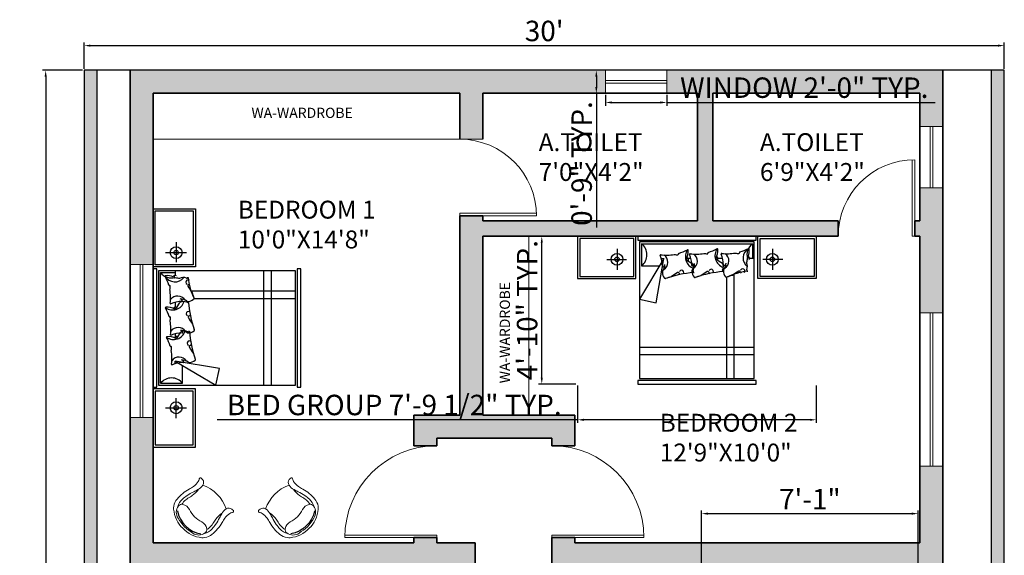
# Model space of a CAD drawing. Units: inches. Extents: x 2700 to 4052, y 1030 to 1872.
# Tile 4 of 8: x 2789 to 3175, y 1632 to 1841. Entities that reach past the tile are written whole.
import ezdxf

# ---------------------------------------------------------------- set-up
doc = ezdxf.new("R2010")
doc.units = ezdxf.units.IN
for name, color, linetype, lineweight in [('A-ANNO-DIMS', 2, 'Continuous', 13), ('A-ANNO-TEXT', 7, 'Continuous', 18), ('A-AREA-IDEN', 7, 'Continuous', 18), ('A-DOOR', 4, 'Continuous', 18), ('A-FLOR-CASE', 8, 'Continuous', 18), ('A-FURN', 8, 'Continuous', 18), ('A-GLAZ', 4, 'Continuous', 18), ('A-WALL', 7, 'Continuous', 35), ('A-WALL-PATT', 7, 'Continuous', 13), ('C-PROP', 7, 'Continuous', 25)]:
    doc.layers.add(name, color=color, linetype=linetype, lineweight=lineweight)
doc.layers.add('C-SITE-PATT', color=252, linetype='Continuous', lineweight=13, true_color=0x939598)
for name, color, linetype in [('FUR', 42, 'Continuous'), ('HA', 9, 'Continuous'), ('HID', 11, 'Continuous'), ('IFF-FURN-DETAIL', 250, 'Continuous'), ('SAN', 5, 'Continuous')]:
    doc.layers.add(name, color=color, linetype=linetype)
doc.styles.get("Standard").update_dxf_attribs({"font": 'arial.ttf'})
doc.dimstyles.new('ISO-25', dxfattribs={"dimtxt": 8, "dimasz": 2.5, "dimexe": 1.25, "dimexo": 0.625, "dimtad": 1, "dimdec": 1, "dimlunit": 3, "dimtxsty": 'Standard', "dimcen": 2.5, "dimclrt": 1, "dimadec": 0, "dimazin": 0, "dimtfac": 1, "dimtdec": 1, "dimtmove": 0, "dimatfit": 3, "dimfxl": 1, "dimarcsym": 0})

# ---------------------------------------------------------------- blocks, each defined once
blk = doc.blocks.new('ILNG95')
for points in [[(120, 308, -0.32971), (51, 384, -0.036099), (50, 422, -0.497733), (75, 439, -0.070621), (96, 429, 0.101868), (133, 414, 0.091794), (259, 412, 0.024114), (351, 433, -0.090294), (638, 458, -0.132412), (775, 407, -0.068618), (816, 368, -0.184346), (943, 0, 1.803905)], [(120, 308, 0.138132), (244, 313, 0.001085), (325, 339, -0.034227), (462, 375, -0.033255), (567, 387, -0.137428), (727, 350, -4.561553)], [(120, 308, 0.138132), (244, 313, 0.001085), (325, 339, -0.034227), (462, 375, -0.033255), (567, 387, -0.137428), (727, 350, -4.561553)], [(235, 308, 0.064243), (394, 307, 0.04414), (433, 315, -0.118032), (643, 329, -6.296816)], [(235, 308, 0.064243), (394, 307, 0.04414), (433, 315, -0.118032), (643, 329, -6.296816)], [(639, 0, 0.078302), (612, 161, -0.233633), (633, 315, -0.28763), (710, 349, -0.317923), (875, 193, -0.032882), (900, 0, 1.140397)], [(639, 0, 0.078302), (612, 161, -0.233633), (633, 315, -0.28763), (710, 349, -0.317923), (875, 193, -0.032882), (900, 0, 1.140397)], [(120, -308, 0.32971), (51, -384, 0.036099), (50, -422, 0.497733), (75, -439, 0.070621), (96, -429, -0.101868), (133, -414, -0.091794), (259, -412, -0.024114), (351, -433, 0.090294), (638, -458, 0.132412), (775, -407, 0.068618), (816, -368, 0.184346), (943, 0, -1.803905)], [(639, 0, -0.078302), (612, -161, 0.233633), (633, -315, 0.28763), (710, -349, 0.317923), (875, -193, 0.032882), (900, 0, -1.140397)], [(639, 0, -0.078302), (612, -161, 0.233633), (633, -315, 0.28763), (710, -349, 0.317923), (875, -193, 0.032882), (900, 0, -1.140397)], [(120, -308, -0.138132), (244, -313, -0.001085), (325, -339, 0.034227), (462, -375, 0.033255), (567, -387, 0.137428), (727, -350, 4.561553)], [(120, -308, -0.138132), (244, -313, -0.001085), (325, -339, 0.034227), (462, -375, 0.033255), (567, -387, 0.137428), (727, -350, 4.561553)], [(235, -308, -0.064243), (394, -307, -0.04414), (433, -315, 0.118032), (643, -329, 6.296816)], [(235, -308, -0.064243), (394, -307, -0.04414), (433, -315, 0.118032), (643, -329, 6.296816)]]:
    blk.add_lwpolyline(points, format="xyb")
blk.add_arc((759, 1), 709, 154.3281, 205.801)
at = {"layer": 'IFF-FURN-DETAIL'}
blk.add_arc((326, -2), 549, 326.8997, 34.6691, dxfattribs=at)
blk.add_arc((326, -2), 549, 326.8997, 34.6691, dxfattribs=at)
blk = doc.blocks.new('A$C73A16738')
at = {"layer": 'FUR'}
for p, q in [((1.15, 2.389), (1.1, 2.164)), ((1.7, 2.064), (1.15, 2.389)), ((1.6, 2.364), (1.6, 2.123)), ((1.9, 2.364), (1.6, 2.364)), ((1.9, 2.364), (1.9, 0.864)), ((1.1, 2.164), (1.7, 2.064)), ((1.7, 2.099), (1.7, 2.064)), ((1.7, 1.695), (1.7, 1.735)), ((1.7, 1.268), (1.7, 1.33)), ((1.7, 0.839), (1.7, 0.904)), ((1.9, 0.864), (1.7, 0.864))]:
    blk.add_line(p, q, dxfattribs=at)
for points in [[(1.428, 2.439), (2, 2.439), (2, 3.229), (1.428, 3.229)], [(1.458, 2.469), (1.97, 2.469), (1.97, 3.199), (1.458, 3.199)], [(0, 2.414), (0, 0.814), (0.05, 0.814), (0.05, 2.414)], [(1.95, 2.414), (1.95, 0.814), (2, 0.814), (2, 2.414)], [(0.075, 0.839), (1.925, 0.839), (1.925, 2.389), (0.075, 2.389)], [(1.428, 0.789), (2, 0.789), (2, 0), (1.428, 0)], [(1.458, 0.759), (1.97, 0.759), (1.97, 0.03), (1.458, 0.03)]]:
    blk.add_lwpolyline(points, close=True, dxfattribs=at)
for centre, start, end in [((1.75, 2.481), 217.7826, 322.2174), ((1.75, 0.748), 37.7826, 105.2747)]:
    blk.add_arc(centre, 0.19, start, end, dxfattribs=at)
at = {"layer": 'HA'}
for p, q in [((0.4, 2.389), (0.4, 0.839)), ((0.5, 2.389), (0.5, 0.839)), ((1.446, 1.214), (0.075, 1.214)), ((1.477, 1.114), (0.075, 1.114))]:
    blk.add_line(p, q, dxfattribs=at)
at = {"layer": 'HID'}
for centre, radius, start, end in [((1.442, 2.042), 0.0144, 131.666, 199.4465), ((0.016, 1.539), 1.498, 4.5852, 19.4465), ((0.016, 1.539), 1.498, 16.386, 19.4465), ((1.51, 1.965), 0.117, 87.3377, 131.666), ((1.515, 2.068), 0.0144, 51.6071, 87.3377), ((1.617, 2.197), 0.15, 231.6071, 269.7845), ((1.65, 2.128), 0.12, 212.7628, 323.8922), ((1.592, 2.074), 0.0072, 92.7363, 208.2985), ((1.628, 2.093), 0.0475, 208.2985, 255.7891), ((1.569, 2.56), 0.48, 272.7363, 290.959), ((1.743, 2.106), 0.0072, 352.7248, 110.959), ((2.348, 2.029), 0.603, 172.7248, 190.2702), ((1.467, 1.966), 0.0144, 196.386, 223.7955), ((0.926, 1.551), 0.667, 29.049, 37.3823), ((1.497, 1.868), 0.0144, 282.6426, 29.049), ((2.038, 1.868), 0.288, 169.4168, 179.3085), ((1.758, 1.872), 0.0072, 179.3085, 290.689), ((1.763, 1.858), 0.0072, 16.2196, 110.689), ((1.51, 1.823), 0.0319, 112.7015, 147.1556), ((1.51, 1.821), 0.0305, 232.3565, 65.7762), ((1.503, 1.839), 0.0144, 102.6426, 112.7015), ((1.722, 1.609), 0.162, 53.8947, 162.3952), ((2.854, 0.961), 1.418, 145.8329, 150.0245), ((3.143, 2.369), 1.611, 202.7018, 202.7206), ((1.683, 1.758), 0.0288, 232.662, 339.1573), ((1.686, 1.753), 0.0072, 38.8315, 145.8329), ((1.788, 1.924), 0.192, 239.9211, 277.124), ((0.088, 1.831), 1.611, 356.4982, 357.2888), ((2.348, 2.029), 0.603, 196.2196, 208.2114), ((1.811, 1.74), 0.0072, 277.124, 28.2114), ((1.811, 1.74), 0.0072, 277.124, 28.2114), ((1.455, 1.642), 0.0144, 131.666, 199.4465), ((0.03, 1.139), 1.498, 4.5852, 19.4465), ((0.03, 1.139), 1.498, 16.386, 19.4465), ((1.524, 1.565), 0.117, 87.3377, 131.666), ((1.524, 1.653), 0.0144, 67.1663, 184.3422), ((1.529, 1.668), 0.0144, 51.6071, 87.3377), ((1.574, 1.774), 0.117, 247.1663, 295.7613), ((1.631, 1.797), 0.15, 231.6071, 269.7845), ((1.663, 1.728), 0.12, 212.7628, 323.8922), ((1.606, 1.674), 0.0072, 92.7363, 208.2985), ((1.642, 1.693), 0.0475, 208.2985, 255.7891), ((1.583, 2.161), 0.48, 272.7363, 290.959), ((1.757, 1.706), 0.0072, 352.7248, 110.959), ((2.362, 1.629), 0.603, 172.7248, 190.2702), ((1.48, 1.566), 0.0144, 196.386, 223.7955), ((0.94, 1.151), 0.667, 29.049, 37.3823), ((1.51, 1.468), 0.0144, 282.6426, 29.049), ((2.052, 1.468), 0.288, 169.4168, 179.3085), ((1.771, 1.472), 0.0072, 179.3085, 290.689), ((1.776, 1.458), 0.0072, 16.2196, 110.689), ((1.523, 1.423), 0.0319, 112.7015, 147.1556), ((1.523, 1.422), 0.0305, 232.3565, 65.7762), ((1.517, 1.44), 0.0144, 102.6426, 112.7015), ((1.736, 1.209), 0.162, 53.8947, 162.3952), ((2.867, 0.561), 1.418, 145.8329, 150.0245), ((3.156, 1.97), 1.611, 202.7018, 202.7206), ((1.697, 1.359), 0.0288, 232.662, 339.1573), ((1.7, 1.353), 0.0072, 38.8315, 145.8329), ((1.802, 1.524), 0.192, 239.9211, 277.124), ((0.102, 1.431), 1.611, 356.4982, 357.2888), ((2.362, 1.629), 0.603, 196.2196, 208.2114), ((1.825, 1.34), 0.0072, 277.124, 28.2114), ((1.825, 1.34), 0.0072, 277.124, 28.2114), ((1.46, 1.216), 0.0144, 131.666, 199.4465), ((0.688, 0.841), 0.844, 6.224, 26.0326), ((0.034, 0.713), 1.498, 16.386, 19.4465), ((1.529, 1.139), 0.117, 87.3377, 131.666), ((1.537, 1.254), 0.0144, 67.1663, 184.3422), ((1.533, 1.242), 0.0144, 51.6071, 87.3377), ((1.635, 1.371), 0.15, 231.6071, 269.7845), ((1.588, 1.374), 0.117, 247.1663, 295.7613), ((1.668, 1.302), 0.12, 212.7628, 323.8922), ((1.611, 1.248), 0.0072, 92.7363, 208.2985), ((1.646, 1.267), 0.0475, 208.2985, 255.7891), ((1.588, 1.734), 0.48, 272.7363, 290.959), ((1.762, 1.28), 0.0072, 352.7248, 110.959), ((2.367, 1.203), 0.603, 172.7248, 190.2702), ((1.485, 1.14), 0.0144, 196.386, 223.7955), ((0.945, 0.725), 0.667, 29.049, 37.3823), ((2.056, 1.042), 0.288, 169.4168, 179.3085), ((1.528, 0.997), 0.0319, 112.7015, 147.1556), ((1.528, 0.995), 0.0305, 232.3565, 65.7762), ((1.521, 1.013), 0.0144, 102.6426, 112.7015), ((1.515, 1.042), 0.0144, 282.6426, 29.049), ((1.542, 0.927), 0.0144, 67.1663, 184.3422), ((1.593, 1.048), 0.117, 247.1663, 295.7613), ((1.705, 0.84), 0.15, 29.3598, 142.4281), ((1.581, 0.528), 0.419, 73.7524, 81.4605), ((1.705, 0.927), 0.0072, 38.8315, 145.8329), ((1.776, 1.046), 0.0072, 179.3085, 290.689), ((1.781, 1.032), 0.0072, 16.2196, 110.689), ((2.367, 1.203), 0.603, 196.2196, 208.2114), ((3.161, 1.543), 1.611, 202.7018, 202.7206), ((1.702, 0.932), 0.0288, 232.662, 339.1573), ((0.106, 1.005), 1.611, 356.4982, 357.2888), ((1.806, 1.098), 0.192, 246.1093, 277.124), ((1.829, 0.914), 0.0072, 277.124, 28.2114), ((1.829, 0.914), 0.0072, 277.124, 28.2114)]:
    blk.add_arc(centre, radius, start, end, dxfattribs=at)
at = {"layer": 'SAN'}
for p, q in [((1.688, 2.835), (1.688, 2.566)), ((1.832, 2.695), (1.546, 2.695)), ((1.688, 0.454), (1.688, 0.723)), ((1.832, 0.594), (1.546, 0.594))]:
    blk.add_line(p, q, dxfattribs=at)
for centre, radius in [((1.688, 2.695), 0.08), ((1.688, 2.695), 0.03), ((1.688, 0.594), 0.08), ((1.688, 0.594), 0.03)]:
    blk.add_circle(centre, radius, dxfattribs=at)
blk = doc.blocks.new('*D19')
at = {"layer": 'A-ANNO-DIMS', "color": 0, "lineweight": -2, "transparency": 16777216}
for p, q in [((2814.67, 1822.14), (2814.67, 1832.43)), ((2817.17, 1831.18), (3172.17, 1831.18)), ((3174.67, 1822.14), (3174.67, 1832.43))]:
    blk.add_line(p, q, dxfattribs=at)
at = {"layer": 'A-ANNO-DIMS', "color": 0, "transparency": 16777216}
for points in [[(2817.17, 1831.6), (2817.17, 1830.77), (2814.67, 1831.18)], [(3172.17, 1831.6), (3172.17, 1830.77), (3174.67, 1831.18)]]:
    blk.add_solid(points, dxfattribs=at)
at = {"layer": 'Defpoints', "color": 0, "transparency": 16777216}
for p in [(3174.67, 1831.18), (2814.67, 1821.52), (3174.67, 1821.52)]:
    blk.add_point(p, dxfattribs=at)
at = {"layer": 'A-ANNO-DIMS', "color": 0, "transparency": 16777216, "insert": (2994.67, 1835.89), "char_height": 8, "attachment_point": 5}
blk.add_mtext("30'", dxfattribs=at)
blk = doc.blocks.new('*D20')
at = {"layer": 'A-ANNO-DIMS', "color": 0, "lineweight": -2, "transparency": 16777216}
for p, q in [((2814.04, 1821.52), (2798.4, 1821.52)), ((2799.65, 1819.02), (2799.65, 1104.02)), ((2814.04, 1101.52), (2798.4, 1101.52))]:
    blk.add_line(p, q, dxfattribs=at)
at = {"layer": 'A-ANNO-DIMS', "color": 0, "transparency": 16777216}
for points in [[(2799.23, 1819.02), (2800.06, 1819.02), (2799.65, 1821.52)], [(2799.23, 1104.02), (2800.06, 1104.02), (2799.65, 1101.52)]]:
    blk.add_solid(points, dxfattribs=at)
at = {"layer": 'Defpoints', "color": 0, "transparency": 16777216}
for p in [(2814.67, 1821.52), (2799.65, 1101.52), (2814.67, 1101.52)]:
    blk.add_point(p, dxfattribs=at)
at = {"layer": 'A-ANNO-DIMS', "color": 0, "transparency": 16777216, "insert": (2794.94, 1461.52), "char_height": 8, "attachment_point": 5, "rotation": 90}
blk.add_mtext("60'", dxfattribs=at)
blk = doc.blocks.new('DOOR-SWING-36IN')
for p, q in [((-1, 36), (-1, 0)), ((0, 36), (0, 0)), ((0, 0), (-1, 0))]:
    blk.add_line(p, q)
blk.add_arc((0, 0), 36, 90, 180)
blk = doc.blocks.new('DOOR-SWING-30IN')
for p, q in [((-1, 30), (-1, 0)), ((0, 30), (0, 0)), ((0, 0), (-1, 0))]:
    blk.add_line(p, q)
blk.add_arc((0, 0), 30, 90, 180)
blk = doc.blocks.new('WINDOW-24IN')
for p, q in [((-4.5, 12), (4.5, 12)), ((-0.5, -12), (-0.5, 12)), ((0.5, -12), (0.5, 12)), ((-4.5, -12), (4.5, -12))]:
    blk.add_line(p, q)
blk = doc.blocks.new('WINDOW-60IN')
for p, q in [((4.5, 30), (-4.5, 30)), ((-0.5, 30), (-0.5, -30)), ((0.5, 30), (0.5, -30)), ((4.5, -30), (-4.5, -30))]:
    blk.add_line(p, q)
blk = doc.blocks.new('*D68')
at = {"layer": 'A-ANNO-DIMS', "color": 0, "lineweight": -2, "transparency": 16777216}
for p, q in [((3018.67, 1811.89), (3018.67, 1807.67)), ((3042.67, 1811.89), (3042.67, 1807.67)), ((3021.17, 1808.92), (3040.17, 1808.92)), ((3042.67, 1808.92), (3147.65, 1808.92))]:
    blk.add_line(p, q, dxfattribs=at)
at = {"layer": 'A-ANNO-DIMS', "color": 0, "transparency": 16777216}
for points in [[(3021.17, 1809.33), (3021.17, 1808.5), (3018.67, 1808.92)], [(3040.17, 1809.33), (3040.17, 1808.5), (3042.67, 1808.92)]]:
    blk.add_solid(points, dxfattribs=at)
at = {"layer": 'Defpoints', "color": 0, "transparency": 16777216}
for p in [(3018.67, 1812.52), (3042.67, 1812.52), (3042.67, 1808.92)]:
    blk.add_point(p, dxfattribs=at)
at = {"layer": 'A-ANNO-DIMS', "color": 1, "transparency": 16777216, "insert": (3096.41, 1813.68), "char_height": 8, "attachment_point": 5}
blk.add_mtext('WINDOW 2\'-0" TYP.', dxfattribs=at)
blk = doc.blocks.new('*D69')
at = {"layer": 'A-ANNO-DIMS', "color": 0, "lineweight": -2, "transparency": 16777216}
for p, q in [((3018.04, 1821.52), (3013.82, 1821.52)), ((3015.07, 1819.02), (3015.07, 1815.02)), ((3018.04, 1812.52), (3013.82, 1812.52)), ((3015.07, 1812.52), (3015.07, 1760))]:
    blk.add_line(p, q, dxfattribs=at)
at = {"layer": 'A-ANNO-DIMS', "color": 0, "transparency": 16777216}
for points in [[(3014.65, 1819.02), (3015.49, 1819.02), (3015.07, 1821.52)], [(3014.65, 1815.02), (3015.49, 1815.02), (3015.07, 1812.52)]]:
    blk.add_solid(points, dxfattribs=at)
at = {"layer": 'Defpoints', "color": 0, "transparency": 16777216}
for p in [(3018.67, 1821.52), (3015.07, 1812.52), (3018.67, 1812.52)]:
    blk.add_point(p, dxfattribs=at)
at = {"layer": 'A-ANNO-DIMS', "color": 1, "transparency": 16777216, "insert": (3010.36, 1785.01), "char_height": 8, "attachment_point": 5, "rotation": 90}
blk.add_mtext('0\'-9" TYP.', dxfattribs=at)
blk = doc.blocks.new('*D84')
at = {"layer": 'A-ANNO-DIMS', "color": 0, "lineweight": -2, "transparency": 16777216}
for p, q in [((3007.73, 1698.05), (3007.73, 1683.42)), ((3101.11, 1698.05), (3101.11, 1683.42)), ((3007.73, 1684.67), (2866.76, 1684.67)), ((3098.61, 1684.67), (3010.23, 1684.67))]:
    blk.add_line(p, q, dxfattribs=at)
at = {"layer": 'A-ANNO-DIMS', "color": 0, "transparency": 16777216}
for points in [[(3010.23, 1685.08), (3010.23, 1684.25), (3007.73, 1684.67)], [(3098.61, 1685.08), (3098.61, 1684.25), (3101.11, 1684.67)]]:
    blk.add_solid(points, dxfattribs=at)
at = {"layer": 'Defpoints', "color": 0, "transparency": 16777216}
for p in [(3007.73, 1698.67), (3101.11, 1698.67), (3007.73, 1684.67)]:
    blk.add_point(p, dxfattribs=at)
at = {"layer": 'A-ANNO-DIMS', "color": 1, "transparency": 16777216, "insert": (2936, 1689.43), "char_height": 8, "attachment_point": 5}
blk.add_mtext('BED GROUP 7\'-9 1/2" TYP.', dxfattribs=at)
blk = doc.blocks.new('*D85')
at = {"layer": 'A-ANNO-DIMS', "color": 0, "lineweight": -2, "transparency": 16777216}
for p, q in [((3007.11, 1756.52), (2992.48, 1756.52)), ((2993.73, 1701.17), (2993.73, 1754.02)), ((3007.11, 1698.67), (2992.48, 1698.67))]:
    blk.add_line(p, q, dxfattribs=at)
at = {"layer": 'A-ANNO-DIMS', "color": 0, "transparency": 16777216}
for points in [[(2993.31, 1754.02), (2994.14, 1754.02), (2993.73, 1756.52)], [(2993.31, 1701.17), (2994.14, 1701.17), (2993.73, 1698.67)]]:
    blk.add_solid(points, dxfattribs=at)
at = {"layer": 'Defpoints', "color": 0, "transparency": 16777216}
for p in [(2993.73, 1756.52), (3007.73, 1756.52), (3007.73, 1698.67)]:
    blk.add_point(p, dxfattribs=at)
at = {"layer": 'A-ANNO-DIMS', "color": 1, "transparency": 16777216, "insert": (2989.02, 1727.6), "char_height": 8, "attachment_point": 5, "rotation": 90}
blk.add_mtext('4\'-10" TYP.', dxfattribs=at)
blk = doc.blocks.new('*D91')
at = {"layer": 'A-ANNO-DIMS', "color": 0, "lineweight": -2, "transparency": 16777216}
for p, q in [((3056.2, 1628.61), (3056.2, 1649.16)), ((3140.98, 1628.61), (3140.98, 1649.16)), ((3058.7, 1647.91), (3138.48, 1647.91))]:
    blk.add_line(p, q, dxfattribs=at)
at = {"layer": 'A-ANNO-DIMS', "color": 0, "transparency": 16777216}
for points in [[(3058.7, 1648.33), (3058.7, 1647.5), (3056.2, 1647.91)], [(3138.48, 1648.33), (3138.48, 1647.5), (3140.98, 1647.91)]]:
    blk.add_solid(points, dxfattribs=at)
at = {"layer": 'Defpoints', "color": 0, "transparency": 16777216}
for p in [(3140.98, 1647.91), (3056.2, 1627.99), (3140.98, 1627.99)]:
    blk.add_point(p, dxfattribs=at)
at = {"layer": 'A-ANNO-DIMS', "color": 1, "transparency": 16777216, "insert": (3098.59, 1652.55), "char_height": 8, "attachment_point": 5}
blk.add_mtext('7\'-1"', dxfattribs=at)

msp = doc.modelspace()

# ---------------------------------------------------------------- hatches: boundary and pattern name
at = {"layer": 'A-WALL-PATT'}
h = msp.add_hatch(color=256, dxfattribs=at)
h.dxf.hatch_style = 1
h.paths.add_polyline_path([(3150.67, 1539.52), (3141.67, 1539.52), (3141.67, 1479.52), (3150.67, 1479.52)])
h.paths.add_polyline_path([(3150.67, 1666.52), (3141.67, 1666.52), (3141.67, 1636.52), (3006.67, 1636.52), (3006.67, 1638.52), (2997.67, 1638.52), (2997.67, 1627.52), (3114.6, 1627.52, -0.035851), (3118.13, 1627.52), (3141.67, 1627.52), (3141.67, 1599.52), (3150.67, 1599.52)])
h.paths.add_polyline_path([(2841.67, 1537.52), (2832.67, 1537.52), (2832.67, 1486.52), (2841.67, 1486.52), (2841.67, 1501.52), (2923.67, 1501.52), (2923.67, 1507.52), (2841.67, 1507.52)], flags=17)
h.paths.add_polyline_path([(2841.67, 1438.52), (2832.67, 1438.52), (2832.67, 1423.52), (2814.67, 1423.52), (2814.67, 1414.52), (2862.67, 1414.52), (2862.67, 1412.52), (2871.67, 1412.52), (2871.67, 1423.52), (2841.67, 1423.52)])
h.paths.add_polyline_path([(2967.67, 1636.52), (2952.67, 1636.52), (2952.67, 1638.52), (2943.67, 1638.52), (2943.67, 1636.52), (2841.67, 1636.52), (2841.67, 1685.52), (2832.67, 1685.52), (2832.67, 1597.52), (2841.67, 1597.52), (2841.67, 1627.52), (2961.67, 1627.52), (2961.67, 1507.52), (2959.67, 1507.52), (2959.67, 1501.52), (2961.67, 1501.52), (2961.67, 1453.52), (2967.67, 1453.52)])
h.paths.add_polyline_path([(2970.67, 1756.52), (3109.67, 1756.52), (3109.67, 1762.52), (3060.67, 1762.52), (3060.67, 1812.52), (3141.67, 1812.52), (3141.67, 1799.52), (3150.67, 1799.52), (3150.67, 1821.52), (3042.67, 1821.52), (3042.67, 1812.52), (3054.67, 1812.52), (3054.67, 1762.52), (2970.67, 1762.52), (2970.67, 1764.52), (2961.67, 1764.52), (2961.67, 1686.52), (2943.67, 1686.52), (2943.67, 1674.52), (2952.67, 1674.52), (2952.67, 1677.52), (2997.67, 1677.52), (2997.67, 1674.52), (3006.67, 1674.52), (3006.67, 1686.52), (2970.67, 1686.52)])
h.paths.add_polyline_path([(3150.67, 1775.52), (3141.67, 1775.52), (3141.67, 1762.52), (3139.67, 1762.52), (3139.67, 1756.52), (3141.67, 1756.52), (3141.67, 1726.52), (3150.67, 1726.52)], flags=17)
h.paths.add_polyline_path([(3018.67, 1821.52), (2832.67, 1821.52), (2832.67, 1745.52), (2841.67, 1745.52), (2841.67, 1812.52), (2961.67, 1812.52), (2961.67, 1794.52), (2970.67, 1794.52), (2970.67, 1812.52), (3018.67, 1812.52)])
h = msp.add_hatch(color=256, dxfattribs=at)
h.dxf.hatch_style = 1
h.paths.add_polyline_path([(2814.67, 1264.52), (2814.67, 1168.52), (2955.67, 1168.52), (2955.67, 1177.52), (2823.67, 1177.52), (2823.67, 1255.52), (2897.67, 1255.52), (2897.67, 1264.52), (2871.67, 1264.52), (2871.67, 1310.49), (2862.67, 1310.49), (2862.67, 1304.37), (2862.67, 1264.52)])
h.paths.add_polyline_path([(2945.67, 1255.52), (2986.67, 1255.52), (2986.67, 1264.52), (2980.67, 1264.52), (2980.67, 1324.52), (3028.67, 1324.52), (3028.67, 1264.52), (3022.67, 1264.52), (3022.67, 1255.52), (3037.67, 1255.52), (3037.67, 1378.52), (3040.67, 1378.52), (3040.67, 1387.52), (3022.67, 1387.52), (3022.67, 1381.52), (3028.67, 1381.52), (3028.67, 1333.52), (2980.67, 1333.52), (2980.67, 1381.52), (2986.67, 1381.52), (2986.67, 1387.52), (2971.67, 1387.52), (2971.67, 1264.52), (2945.67, 1264.52)])
h.paths.add_polyline_path([(2871.67, 1358.49), (2871.67, 1382.52), (2862.67, 1382.52), (2862.67, 1358.49)])
h.paths.add_polyline_path([(3091.67, 1387.52), (3088.67, 1387.52), (3088.67, 1378.52), (3091.67, 1378.52)])
h.paths.add_polyline_path([(3141.67, 1300.52), (3150.67, 1300.52), (3150.67, 1431.52), (3141.67, 1431.52), (3141.67, 1387.52), (3139.67, 1387.52), (3139.67, 1378.52), (3141.67, 1378.52)])
h.paths.add_polyline_path([(2830.28, 1565.14), (2830.28, 1604.05), (2822.03, 1604.05), (2822.03, 1565.14)], flags=9)
h.paths.add_polyline_path([(2957.35, 1565.68), (2957.35, 1611.46), (2949.11, 1611.46), (2949.11, 1565.68)], flags=9)
h.paths.add_polyline_path([(2983.54, 1697.89), (2983.54, 1743.66), (2975.29, 1743.66), (2975.29, 1697.89)], flags=9)
h.paths.add_polyline_path([(2879.08, 1800.61), (2924.85, 1800.61), (2924.85, 1808.85), (2879.08, 1808.85)], flags=9)
h.paths.add_polyline_path([(2815.49, 1361.72), (2864.45, 1361.72), (2864.45, 1388.34), (2815.49, 1388.34)], flags=9)
h.paths.add_polyline_path([(2904.6, 1318.27), (2953.91, 1318.27), (2953.91, 1344.89), (2904.6, 1344.89)], flags=9)
h.paths.add_polyline_path([(3036.9, 1507.34), (3091.04, 1507.34), (3091.04, 1533.96), (3036.9, 1533.96)], flags=9)
h.paths.add_polyline_path([(2990.4, 1774.23), (3040.41, 1774.23), (3040.41, 1800.84), (2990.4, 1800.84)], flags=9)
h.paths.add_polyline_path([(3076.88, 1774.23), (3126.96, 1774.23), (3126.96, 1800.84), (3076.88, 1800.84)], flags=9)
h.paths.add_polyline_path([(3036.9, 1664.37), (3100.88, 1664.37), (3100.88, 1690.98), (3036.9, 1690.98)], flags=9)
h.paths.add_polyline_path([(2871.85, 1747.79), (2935.82, 1747.79), (2935.82, 1774.41), (2871.85, 1774.41)], flags=9)
h.paths.add_polyline_path([(2871.85, 1590.97), (2935.82, 1590.97), (2935.82, 1617.58), (2871.85, 1617.58)], flags=9)
h.paths.add_polyline_path([(2862.5, 1447.4), (2911.46, 1447.4), (2911.46, 1474.01), (2862.5, 1474.01)], flags=9)
at = {"layer": 'C-SITE-PATT'}
h = msp.add_hatch(color=256, dxfattribs=at)
h.dxf.hatch_style = 1
h.paths.add_polyline_path([(2819.67, 1821.52), (2814.67, 1821.52), (2814.67, 1423.52), (2819.67, 1423.52)])
h.paths.add_polyline_path([(3037.67, 1108.52), (2819.67, 1108.52), (2819.67, 1168.52), (2814.67, 1168.52), (2814.67, 1101.52), (3037.67, 1101.52)])
h.paths.add_polyline_path([(3174.67, 1821.52), (3169.67, 1821.52), (3169.67, 1108.52), (3157.67, 1108.52), (3157.67, 1101.52), (3174.67, 1101.52)])

# ---------------------------------------------------------------- linework, layer by layer
at = {"layer": 'A-FLOR-CASE'}
for p, q in [((2970.67, 1794.52), (2841.67, 1794.52)), ((2988.67, 1756.52), (2988.67, 1686.52))]:
    msp.add_line(p, q, dxfattribs=at)
at = {"layer": 'A-WALL'}
for p, q in [((2832.67, 1821.52), (2832.67, 1423.52)), ((3150.67, 1300.52), (3150.67, 1821.52)), ((2841.67, 1812.52), (2841.67, 1636.52)), ((2961.67, 1812.52), (2841.67, 1812.52)), ((2961.67, 1812.52), (2961.67, 1794.52)), ((2970.67, 1812.52), (2970.67, 1794.52)), ((3054.67, 1812.52), (2970.67, 1812.52)), ((3054.67, 1812.52), (3054.67, 1762.52)), ((3141.67, 1812.52), (3060.67, 1812.52)), ((3060.67, 1812.52), (3060.67, 1762.52)), ((3141.67, 1762.52), (3141.67, 1812.52)), ((2970.67, 1764.52), (2961.67, 1764.52)), ((2961.67, 1764.52), (2961.67, 1686.52)), ((2970.67, 1764.52), (2970.67, 1762.52)), ((3054.67, 1762.52), (2970.67, 1762.52)), ((3109.67, 1762.52), (3060.67, 1762.52)), ((3109.67, 1756.52), (3109.67, 1762.52)), ((3141.67, 1762.52), (3139.67, 1762.52)), ((3139.67, 1756.52), (3139.67, 1762.52)), ((2970.67, 1756.52), (2970.67, 1686.52)), ((3109.67, 1756.52), (2970.67, 1756.52)), ((3141.67, 1756.52), (3139.67, 1756.52)), ((3141.67, 1636.52), (3141.67, 1756.52)), ((2943.67, 1686.52), (2943.67, 1674.52)), ((2961.67, 1686.52), (2943.67, 1686.52)), ((3006.67, 1686.52), (2970.67, 1686.52)), ((3006.67, 1686.52), (3006.67, 1674.52)), ((2997.67, 1677.52), (2952.67, 1677.52)), ((2952.67, 1677.52), (2952.67, 1674.52)), ((2997.67, 1677.52), (2997.67, 1674.52)), ((2952.67, 1674.52), (2943.67, 1674.52)), ((3006.67, 1674.52), (2997.67, 1674.52)), ((2952.67, 1638.52), (2943.67, 1638.52)), ((2943.67, 1638.52), (2943.67, 1636.52)), ((2952.67, 1638.52), (2952.67, 1636.52)), ((3006.67, 1638.52), (2997.67, 1638.52)), ((2997.67, 1638.52), (2997.67, 1627.52)), ((3006.67, 1638.52), (3006.67, 1636.52)), ((2943.67, 1636.52), (2841.67, 1636.52)), ((2967.67, 1636.52), (2952.67, 1636.52)), ((2967.67, 1636.52), (2967.67, 1453.52)), ((3141.67, 1636.52), (3006.67, 1636.52))]:
    msp.add_line(p, q, dxfattribs=at)
at = {"layer": 'C-PROP'}
for p, q in [((2819.67, 1821.52), (2819.67, 1423.52)), ((3169.67, 1108.52), (3169.67, 1821.52))]:
    msp.add_line(p, q, dxfattribs=at)
msp.add_lwpolyline([(3157.67, 1101.52), (3174.67, 1101.52), (3174.67, 1821.52), (2814.67, 1821.52), (2814.67, 1101.52), (3037.67, 1101.52)], dxfattribs=at)

# ---------------------------------------------------------------- block references
at = {"layer": 'A-DOOR'}
for name, p, rotation in [('DOOR-SWING-30IN', (2961.67, 1764.52), 270.0000000000011), ('DOOR-SWING-36IN', (2997.67, 1638.52), 270.0000000000012)]:
    msp.add_blockref(name, p, dxfattribs=dict(at, rotation=rotation))
msp.add_blockref('DOOR-SWING-30IN', (3139.67, 1756.52), dxfattribs=at)
at = {"layer": 'A-DOOR', "extrusion": (0, 0, -1), "zscale": -1, "rotation": 270.0000000000012}
msp.add_blockref('DOOR-SWING-36IN', (-2952.67, 1638.52), dxfattribs=at)
at = {"layer": 'A-FURN'}
for name, p, xscale, yscale, zscale, rotation in [('A$C73A16738', (2899.51, 1767.32), 28.92215291203286, 28.92215291203286, 28.92215291203286, 180), ('A$C73A16738', (3101.11, 1698.67), 28.92215291203286, 28.92215291203286, 28.92215291203286, 89.99999999999999), ('ILNG95', (2867.53, 1656.22), 0.0212192471586889, 0.0212192471586889, 0.0212192471586889, 224.6051083961163), ('ILNG95', (2888.47, 1656.22), -0.0212192471586889, 0.0212192471586889, 0.0212192471586889, 135.3948916038836)]:
    msp.add_blockref(name, p, dxfattribs=dict(at, xscale=xscale, yscale=yscale, zscale=zscale, rotation=rotation))
at = {"layer": 'A-GLAZ'}
for name, p, rotation in [('WINDOW-24IN', (3030.67, 1817.02), 270.0000000000046), ('WINDOW-60IN', (3146.17, 1696.52), 180)]:
    msp.add_blockref(name, p, dxfattribs=dict(at, rotation=rotation))
for name, p in [('WINDOW-24IN', (3146.17, 1787.52)), ('WINDOW-60IN', (2837.17, 1715.52))]:
    msp.add_blockref(name, p, dxfattribs=at)

# ---------------------------------------------------------------- texts
at = {"layer": 'A-ANNO-TEXT', "insert": (2880.15, 1806.86), "char_height": 4, "attachment_point": 1}
msp.add_mtext_dynamic_manual_height_columns('WA-WARDROBE', width=29.5334, gutter_width=12.5, heights=[0], dxfattribs=at)
at = {"layer": 'A-ANNO-TEXT', "insert": (2977.28, 1698.96), "char_height": 4, "attachment_point": 1, "rotation": 90}
msp.add_mtext_dynamic_manual_height_columns('WA-WARDROBE', width=29.5334, gutter_width=12.5, heights=[0], dxfattribs=at)
at = {"layer": 'A-AREA-IDEN', "char_height": 7, "attachment_point": 1}
for s, insert in [('{\\fTimes New Roman|b0|i0|c0|p18;A.TOILET\\P7\'0"X4\'2"}', (2992.53, 1796.88)), ('{\\fTimes New Roman|b0|i0|c0|p18;A.TOILET\\P6\'9"X4\'2"}', (3079.08, 1796.88)), ('{\\fTimes New Roman|b0|i0|c0|p18;BEDROOM 1\\P10\'0"X14\'8"}', (2874.81, 1770.45)), ('{\\fTimes New Roman|b0|i0|c0|p18;BEDROOM 2\\P12\'9"X10\'0"}', (3039.86, 1687.02))]:
    msp.add_mtext_dynamic_manual_height_columns(s, width=61.0557, gutter_width=12.5, heights=[0], dxfattribs=dict(at, insert=insert))

# ---------------------------------------------------------------- dimensions: what is measured, and where the dimension line sits
at = {"layer": 'A-ANNO-DIMS'}
for base, p1, p2, override, picture, middle in [((3174.67, 1831.18), (2814.67, 1821.52), (3174.67, 1821.52), {"dimclrd": 0, "dimclre": 0, "dimclrt": 0}, '*D19', (2994.67, 1835.89)), ((3140.98, 1647.91), (3056.2, 1627.99), (3140.98, 1627.99), {"dimdec": 1, "dimlfac": 1, "dimrnd": 0, "dimzin": 1, "dimdsep": 46, "dimlunit": 4, "dimfrac": 2}, '*D91', (3098.59, 1652.55))]:
    dim = msp.add_linear_dim(base=base, p1=p1, p2=p2, dimstyle='ISO-25', override=override, dxfattribs=at)
    dim.commit()
    dim.dimension.update_dxf_attribs({"geometry": picture, "text_midpoint": middle})
for base, p1, p2, angle, text, picture, middle in [((3042.67, 1808.92), (3018.67, 1812.52), (3042.67, 1812.52), 0, 'WINDOW <> TYP.', '*D68', (3096.41, 1813.68)), ((3015.07, 1812.52), (3018.67, 1821.52), (3018.67, 1812.52), 270, '<> TYP.', '*D69', (3010.36, 1785.01)), ((2993.7275, 1756.5174), (3007.7345, 1698.6731), (3007.7345, 1756.5174), 90, '<> TYP.', '*D85', (2989.0179, 1727.5952)), ((3007.73, 1684.67), (3101.11, 1698.67), (3007.73, 1698.67), 180, 'BED GROUP <> TYP.', '*D84', (2936, 1689.43))]:
    dim = msp.add_linear_dim(base=base, p1=p1, p2=p2, angle=angle, text=text, dimstyle='ISO-25', override={"dimdec": 1, "dimlfac": 1, "dimrnd": 0, "dimzin": 1, "dimdsep": 46, "dimlunit": 4, "dimfrac": 2}, dxfattribs=at)
    dim.commit()
    dim.dimension.update_dxf_attribs({"geometry": picture, "text_midpoint": middle})
dim = msp.add_linear_dim(base=(2799.65, 1101.52), p1=(2814.67, 1821.52), p2=(2814.67, 1101.52), angle=90, dimstyle='ISO-25', override={"dimclrd": 0, "dimclre": 0, "dimclrt": 0}, dxfattribs=at)
dim.commit()
dim.dimension.update_dxf_attribs({"geometry": '*D20', "text_midpoint": (2794.94, 1461.52)})

doc.saveas('drawing.dxf')
